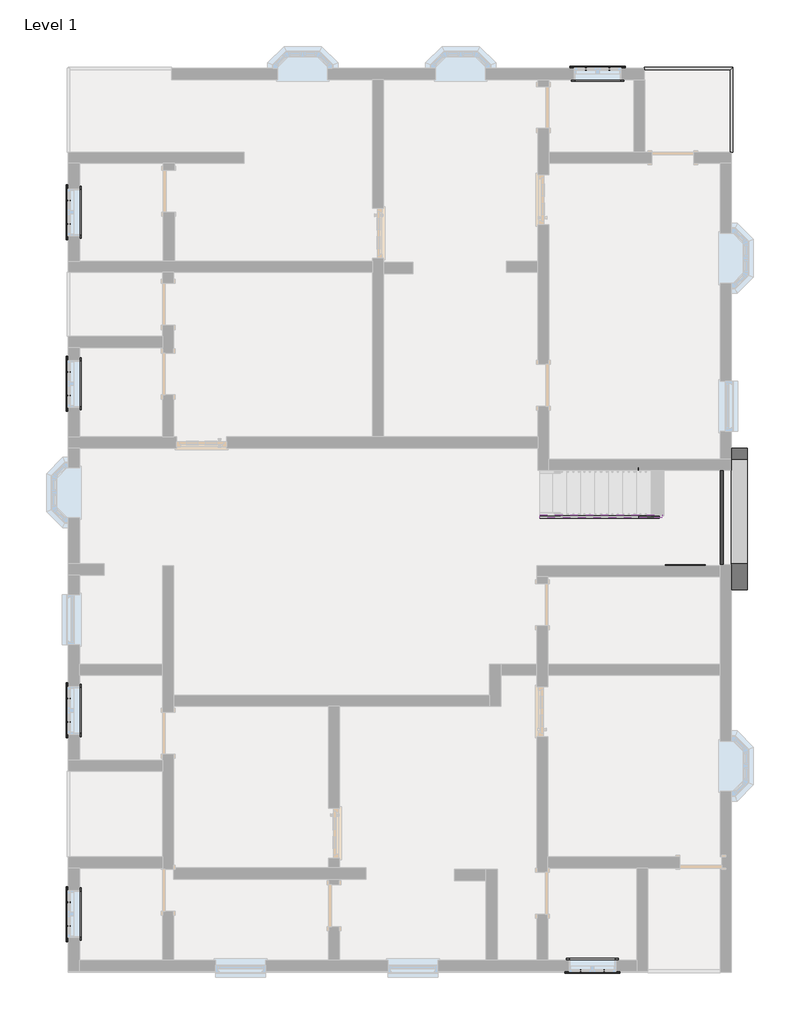
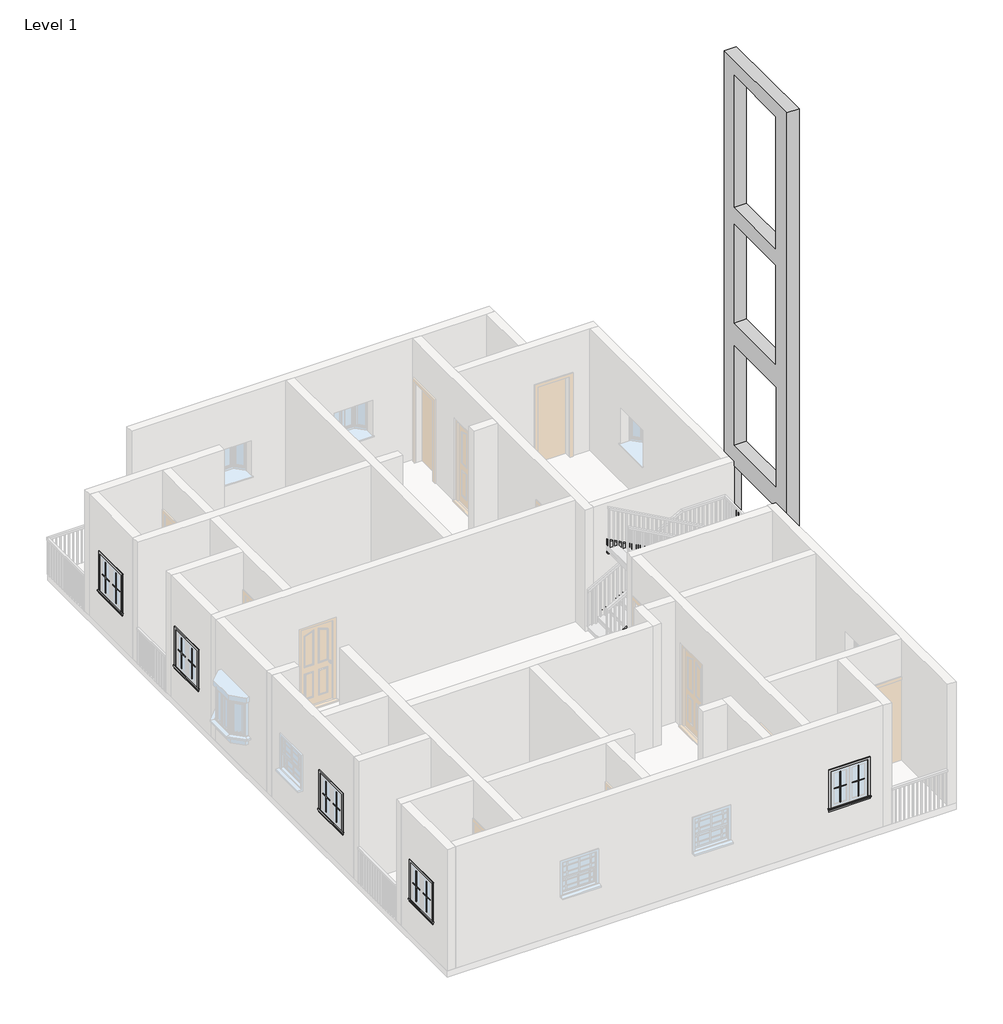
# One storey, part 4 of 4: 25 proxies, 5 members, 1 railing.
"""IFC4 building model written with IfcOpenShell, lengths in millimetres."""

from ifc_helpers import new_model, si_unit, frame, origin, origin_with_axes, place, context, project, spatial, polyline, outline, extrude, faceted_brep, transform, mapped, element, save
from components import generic_models_1_generic_models_1_8cf75778, muntin_pattern_2x2_muntin_pattern_2x2_b3fe6957, muntin_pattern_2x2_muntin_pattern_2x2_3e0ecaf2, trim_window_exterior_flat_with_sill_41619996, trim_window_interior_flat_picture_frame_51c85655

model = new_model("IFC4")

# Units and contexts
model_context = context("Model", 3, world=origin())
ifc_project = project(units=[si_unit("LENGTHUNIT", "METRE", prefix="MILLI")], contexts=[model_context])

# Site, building, storey
site = spatial("IfcSite", under=ifc_project)
building = spatial("IfcBuilding", under=site)
storey = spatial("IfcBuildingStorey", under=building, Name="Level 1", Elevation=0.0)

# Proxies
placement = place(None, origin())
generic_models_1_generic_models_1_shape = generic_models_1_generic_models_1_8cf75778(model_context)
element("IfcBuildingElementProxy", 1, Name="Generic Models 1 : Generic Models 1", ObjectType="Generic Models 1 : Generic Models 1", at=placement, inside=storey, context=model_context, shape_type="MappedRepresentation", body=[
    mapped(generic_models_1_generic_models_1_shape, transform((0.0, 0.0, 0.0), x_axis=(1.0, 0.0, 0.0), y_axis=(0.0, 1.0, 0.0), z_axis=(0.0, 0.0, 1.0))),
])
muntin_pattern_2x2_muntin_pattern_2x2_shape = muntin_pattern_2x2_muntin_pattern_2x2_b3fe6957(model_context)
element("IfcBuildingElementProxy", 2, Name="Muntin Pattern_2x2 : Muntin Pattern_2x2", ObjectType="Muntin Pattern_2x2 : Muntin Pattern_2x2", at=placement, inside=storey, context=model_context, shape_type="MappedRepresentation", body=[
    mapped(muntin_pattern_2x2_muntin_pattern_2x2_shape, transform((-7038.4808717, 5489.0318597, 984.25), x_axis=(0.0, 1.0, 0.0), y_axis=(-1.0, 0.0, 0.0), z_axis=(0.0, 0.0, 1.0))),
])
element("IfcBuildingElementProxy", 3, Name="Muntin Pattern_2x2 : Muntin Pattern_2x2", ObjectType="Muntin Pattern_2x2 : Muntin Pattern_2x2", at=placement, inside=storey, context=model_context, shape_type="MappedRepresentation", body=[
    mapped(muntin_pattern_2x2_muntin_pattern_2x2_shape, transform((-7038.4808717, 2366.9422293, 984.25), x_axis=(0.0, 1.0, 0.0), y_axis=(-1.0, 0.0, 0.0), z_axis=(0.0, 0.0, 1.0))),
])
element("IfcBuildingElementProxy", 4, Name="Muntin Pattern_2x2 : Muntin Pattern_2x2", ObjectType="Muntin Pattern_2x2 : Muntin Pattern_2x2", at=placement, inside=storey, context=model_context, shape_type="MappedRepresentation", body=[
    mapped(muntin_pattern_2x2_muntin_pattern_2x2_shape, transform((2376.9816283, 8312.1297293, 984.25), x_axis=(1.0, 0.0, 0.0), y_axis=(0.0, 1.0, 0.0), z_axis=(0.0, 0.0, 1.0))),
])
element("IfcBuildingElementProxy", 5, Name="Muntin Pattern_2x2 : Muntin Pattern_2x2", ObjectType="Muntin Pattern_2x2 : Muntin Pattern_2x2", at=placement, inside=storey, context=model_context, shape_type="MappedRepresentation", body=[
    mapped(muntin_pattern_2x2_muntin_pattern_2x2_shape, transform((2710.3566283, -8102.6202707, 984.25), x_axis=(-1.0, 0.0, 0.0), y_axis=(0.0, -1.0, 0.0), z_axis=(0.0, 0.0, 1.0))),
])
element("IfcBuildingElementProxy", 6, Name="Muntin Pattern_2x2 : Muntin Pattern_2x2", ObjectType="Muntin Pattern_2x2 : Muntin Pattern_2x2", at=placement, inside=storey, context=model_context, shape_type="MappedRepresentation", body=[
    mapped(muntin_pattern_2x2_muntin_pattern_2x2_shape, transform((-7038.4808717, -7285.0577707, 984.25), x_axis=(0.0, 1.0, 0.0), y_axis=(-1.0, 0.0, 0.0), z_axis=(0.0, 0.0, 1.0))),
])
element("IfcBuildingElementProxy", 7, Name="Muntin Pattern_2x2 : Muntin Pattern_2x2", ObjectType="Muntin Pattern_2x2 : Muntin Pattern_2x2", at=placement, inside=storey, context=model_context, shape_type="MappedRepresentation", body=[
    mapped(muntin_pattern_2x2_muntin_pattern_2x2_shape, transform((-7038.4808717, -3576.6577707, 984.25), x_axis=(0.0, 1.0, 0.0), y_axis=(-1.0, 0.0, 0.0), z_axis=(0.0, 0.0, 1.0))),
])
muntin_pattern_2x2_muntin_pattern_2x2_2_shape = muntin_pattern_2x2_muntin_pattern_2x2_3e0ecaf2(model_context)
element("IfcBuildingElementProxy", 8, Name="Muntin Pattern_2x2 : Muntin Pattern_2x2", ObjectType="Muntin Pattern_2x2 : Muntin Pattern_2x2", at=placement, inside=storey, context=model_context, shape_type="MappedRepresentation", body=[
    mapped(muntin_pattern_2x2_muntin_pattern_2x2_2_shape, transform((-7038.4808717, 5917.6568597, 984.25), x_axis=(0.0, -1.0, 0.0), y_axis=(1.0, 0.0, 0.0), z_axis=(0.0, 0.0, 1.0))),
])
element("IfcBuildingElementProxy", 9, Name="Muntin Pattern_2x2 : Muntin Pattern_2x2", ObjectType="Muntin Pattern_2x2 : Muntin Pattern_2x2", at=placement, inside=storey, context=model_context, shape_type="MappedRepresentation", body=[
    mapped(muntin_pattern_2x2_muntin_pattern_2x2_2_shape, transform((-7038.4808717, 2795.5672293, 984.25), x_axis=(0.0, -1.0, 0.0), y_axis=(1.0, 0.0, 0.0), z_axis=(0.0, 0.0, 1.0))),
])
element("IfcBuildingElementProxy", 10, Name="Muntin Pattern_2x2 : Muntin Pattern_2x2", ObjectType="Muntin Pattern_2x2 : Muntin Pattern_2x2", at=placement, inside=storey, context=model_context, shape_type="MappedRepresentation", body=[
    mapped(muntin_pattern_2x2_muntin_pattern_2x2_2_shape, transform((2805.6066283, 8312.1297293, 984.25), x_axis=(-1.0, 0.0, 0.0), y_axis=(0.0, -1.0, 0.0), z_axis=(0.0, 0.0, 1.0))),
])
element("IfcBuildingElementProxy", 11, Name="Muntin Pattern_2x2 : Muntin Pattern_2x2", ObjectType="Muntin Pattern_2x2 : Muntin Pattern_2x2", at=placement, inside=storey, context=model_context, shape_type="MappedRepresentation", body=[
    mapped(muntin_pattern_2x2_muntin_pattern_2x2_2_shape, transform((2281.7316283, -8102.6202707, 984.25), x_axis=(1.0, 0.0, 0.0), y_axis=(0.0, 1.0, 0.0), z_axis=(0.0, 0.0, 1.0))),
])
element("IfcBuildingElementProxy", 12, Name="Muntin Pattern_2x2 : Muntin Pattern_2x2", ObjectType="Muntin Pattern_2x2 : Muntin Pattern_2x2", at=placement, inside=storey, context=model_context, shape_type="MappedRepresentation", body=[
    mapped(muntin_pattern_2x2_muntin_pattern_2x2_2_shape, transform((-7038.4808717, -6856.4327707, 984.25), x_axis=(0.0, -1.0, 0.0), y_axis=(1.0, 0.0, 0.0), z_axis=(0.0, 0.0, 1.0))),
])
element("IfcBuildingElementProxy", 13, Name="Muntin Pattern_2x2 : Muntin Pattern_2x2", ObjectType="Muntin Pattern_2x2 : Muntin Pattern_2x2", at=placement, inside=storey, context=model_context, shape_type="MappedRepresentation", body=[
    mapped(muntin_pattern_2x2_muntin_pattern_2x2_2_shape, transform((-7038.4808717, -3148.0327707, 984.25), x_axis=(0.0, -1.0, 0.0), y_axis=(1.0, 0.0, 0.0), z_axis=(0.0, 0.0, 1.0))),
])
trim_window_exterior_flat_with_sill_shape = trim_window_exterior_flat_with_sill_41619996(model_context)
element("IfcBuildingElementProxy", 14, Name="Trim-Window-Exterior-Flat : with Sill", ObjectType="Trim-Window-Exterior-Flat : with Sill", at=placement, inside=storey, context=model_context, shape_type="MappedRepresentation", body=[
    mapped(trim_window_exterior_flat_with_sill_shape, transform((-7048.0058717, 5703.3443597, 1828.8), x_axis=(0.0, -1.0, 0.0), y_axis=(0.0, 0.0, 1.0), z_axis=(-1.0, 0.0, 0.0))),
])
element("IfcBuildingElementProxy", 15, Name="Trim-Window-Exterior-Flat : with Sill", ObjectType="Trim-Window-Exterior-Flat : with Sill", at=placement, inside=storey, context=model_context, shape_type="MappedRepresentation", body=[
    mapped(trim_window_exterior_flat_with_sill_shape, transform((-7048.0058717, 2581.2547293, 1828.8), x_axis=(0.0, -1.0, 0.0), y_axis=(0.0, 0.0, 1.0), z_axis=(-1.0, 0.0, 0.0))),
])
element("IfcBuildingElementProxy", 16, Name="Trim-Window-Exterior-Flat : with Sill", ObjectType="Trim-Window-Exterior-Flat : with Sill", at=placement, inside=storey, context=model_context, shape_type="MappedRepresentation", body=[
    mapped(trim_window_exterior_flat_with_sill_shape, transform((2591.2941283, 8321.6547293, 1828.8), x_axis=(-1.0, 0.0, 0.0), y_axis=(0.0, 0.0, 1.0), z_axis=(0.0, 1.0, 0.0))),
])
element("IfcBuildingElementProxy", 17, Name="Trim-Window-Exterior-Flat : with Sill", ObjectType="Trim-Window-Exterior-Flat : with Sill", at=placement, inside=storey, context=model_context, shape_type="MappedRepresentation", body=[
    mapped(trim_window_exterior_flat_with_sill_shape, transform((2496.0441283, -8112.1452707, 1828.8), x_axis=(1.0, 0.0, 0.0), y_axis=(0.0, 0.0, 1.0), z_axis=(0.0, -1.0, 0.0))),
])
element("IfcBuildingElementProxy", 18, Name="Trim-Window-Exterior-Flat : with Sill", ObjectType="Trim-Window-Exterior-Flat : with Sill", at=placement, inside=storey, context=model_context, shape_type="MappedRepresentation", body=[
    mapped(trim_window_exterior_flat_with_sill_shape, transform((-7048.0058717, -7070.7452707, 1828.8), x_axis=(0.0, -1.0, 0.0), y_axis=(0.0, 0.0, 1.0), z_axis=(-1.0, 0.0, 0.0))),
])
element("IfcBuildingElementProxy", 19, Name="Trim-Window-Exterior-Flat : with Sill", ObjectType="Trim-Window-Exterior-Flat : with Sill", at=placement, inside=storey, context=model_context, shape_type="MappedRepresentation", body=[
    mapped(trim_window_exterior_flat_with_sill_shape, transform((-7048.0058717, -3362.3452707, 1828.8), x_axis=(0.0, -1.0, 0.0), y_axis=(0.0, 0.0, 1.0), z_axis=(-1.0, 0.0, 0.0))),
])
trim_window_interior_flat_picture_frame_shape = trim_window_interior_flat_picture_frame_51c85655(model_context)
element("IfcBuildingElementProxy", 20, Name="Trim-Window-Interior-Flat : Picture Frame", ObjectType="Trim-Window-Interior-Flat : Picture Frame", at=placement, inside=storey, context=model_context, shape_type="MappedRepresentation", body=[
    mapped(trim_window_interior_flat_picture_frame_shape, transform((-6844.8058717, 5703.3443597, 1828.8), x_axis=(0.0, 1.0, 0.0), y_axis=(0.0, 0.0, 1.0), z_axis=(1.0, 0.0, 0.0))),
])
element("IfcBuildingElementProxy", 21, Name="Trim-Window-Interior-Flat : Picture Frame", ObjectType="Trim-Window-Interior-Flat : Picture Frame", at=placement, inside=storey, context=model_context, shape_type="MappedRepresentation", body=[
    mapped(trim_window_interior_flat_picture_frame_shape, transform((-6844.8058717, 2581.2547293, 1828.8), x_axis=(0.0, 1.0, 0.0), y_axis=(0.0, 0.0, 1.0), z_axis=(1.0, 0.0, 0.0))),
])
element("IfcBuildingElementProxy", 22, Name="Trim-Window-Interior-Flat : Picture Frame", ObjectType="Trim-Window-Interior-Flat : Picture Frame", at=placement, inside=storey, context=model_context, shape_type="MappedRepresentation", body=[
    mapped(trim_window_interior_flat_picture_frame_shape, transform((2591.2941283, 8118.4547293, 1828.8), x_axis=(1.0, 0.0, 0.0), y_axis=(0.0, 0.0, 1.0), z_axis=(0.0, -1.0, 0.0))),
])
element("IfcBuildingElementProxy", 23, Name="Trim-Window-Interior-Flat : Picture Frame", ObjectType="Trim-Window-Interior-Flat : Picture Frame", at=placement, inside=storey, context=model_context, shape_type="MappedRepresentation", body=[
    mapped(trim_window_interior_flat_picture_frame_shape, transform((2496.0441283, -7908.9452707, 1828.8), x_axis=(-1.0, 0.0, 0.0), y_axis=(0.0, 0.0, 1.0), z_axis=(0.0, 1.0, 0.0))),
])
element("IfcBuildingElementProxy", 24, Name="Trim-Window-Interior-Flat : Picture Frame", ObjectType="Trim-Window-Interior-Flat : Picture Frame", at=placement, inside=storey, context=model_context, shape_type="MappedRepresentation", body=[
    mapped(trim_window_interior_flat_picture_frame_shape, transform((-6844.8058717, -7070.7452707, 1828.8), x_axis=(0.0, 1.0, 0.0), y_axis=(0.0, 0.0, 1.0), z_axis=(1.0, 0.0, 0.0))),
])
element("IfcBuildingElementProxy", 25, Name="Trim-Window-Interior-Flat : Picture Frame", ObjectType="Trim-Window-Interior-Flat : Picture Frame", at=placement, inside=storey, context=model_context, shape_type="MappedRepresentation", body=[
    mapped(trim_window_interior_flat_picture_frame_shape, transform((-6844.8058717, -3362.3452707, 1828.8), x_axis=(0.0, 1.0, 0.0), y_axis=(0.0, 0.0, 1.0), z_axis=(1.0, 0.0, 0.0))),
])

# Members
element("IfcMember", 26, ObjectType="Stringer - 2\" Width", at=placement, inside=storey, context=model_context, shape_type="SweptSolid", body=[
    extrude(outline(polyline([(210.6757607, 1537.1941283), (0.0, 1537.1941283), (0.0, 1786.1766781), (1447.8, 4407.1563102), (1447.8, 3776.7834593), (210.6757607, 1537.1941283)])), frame((0.0, 1006.4547293, 0.0), z_axis=(0.0, 1.0, 0.0), x_axis=(0.0, 0.0, 1.0)), (0.0, 0.0, 1.0), 50.8),
])
element("IfcMember", 27, ObjectType="Stringer - 2\" Width", at=placement, inside=storey, context=model_context, shape_type="SweptSolid", body=[
    extrude(outline(polyline([(4826.4941283, 1057.2547293), (4877.2941283, 1057.2547293), (4877.2941283, -714.2964201), (4826.4941283, -714.2964201), (4826.4941283, 1057.2547293)])), frame((0.0, 0.0, 1143.0), z_axis=(0.0, 0.0, 1.0), x_axis=(1.0, 0.0, 0.0)), (0.0, 0.0, 1.0), 304.8),
])
element("IfcMember", 28, ObjectType="Stringer - 2\" Width", at=placement, inside=storey, context=model_context, shape_type="SweptSolid", body=[
    extrude(outline(polyline([(1143.0, 4555.0346706), (2810.0215532, 1537.1941283), (2461.8106009, 1537.1941283), (1143.0, 3924.6618197), (1143.0, 4555.0346706)])), frame((0.0, -765.0964201, 0.0), z_axis=(0.0, 1.0, 0.0), x_axis=(0.0, 0.0, 1.0)), (0.0, 0.0, 1.0), 50.8),
])
element("IfcMember", 29, ObjectType="Stringer - 2\" Width", at=placement, inside=storey, context=model_context, shape_type="SweptSolid", body=[
    extrude(outline(polyline([(210.6757607, 1537.1941283), (0.0, 1537.1941283), (0.0, 1786.1766781), (1065.4963497, 3715.0648053), (1413.7073019, 3715.0648053), (210.6757607, 1537.1941283)])), frame((0.0, 130.1547293, 0.0), z_axis=(0.0, 1.0, 0.0), x_axis=(0.0, 0.0, 1.0)), (0.0, 0.0, 1.0), 50.8),
])
element("IfcMember", 30, ObjectType="Stringer - 2\" Width", at=placement, inside=storey, context=model_context, shape_type="SweptSolid", body=[
    extrude(outline(polyline([(1230.7177047, 3765.8648053), (1578.928657, 3765.8648053), (2810.0215532, 1537.1941283), (2461.8106009, 1537.1941283), (1230.7177047, 3765.8648053)])), frame((0.0, 142.8547293, 0.0), z_axis=(0.0, 1.0, 0.0), x_axis=(0.0, 0.0, 1.0)), (0.0, 0.0, 1.0), 50.8),
])

# Railing
element("IfcRailing", 31, ObjectType="Handrail - Rectangular", at=placement, inside=storey, context=model_context, shape_type="SolidModel", body=[
    faceted_brep([(3442.1941283, 8347.0547293, 914.4), (3442.1941283, 8347.0547293, 863.6), (3442.1941283, 8296.2547293, 863.6), (3442.1941283, 8296.2547293, 914.4), (5055.0941283, 8347.0547293, 914.4), (5055.0941283, 8347.0547293, 863.6), (5004.2941283, 8296.2547293, 863.6), (5004.2941283, 8296.2547293, 914.4), (5055.0941283, 6797.6547293, 914.4), (5004.2941283, 6797.6547293, 914.4), (5004.2941283, 6797.6547293, 863.6), (5055.0941283, 6797.6547293, 863.6)], [[[0, 1, 2, 3]], [[1, 0, 4, 5]], [[2, 1, 5, 6]], [[3, 2, 6, 7]], [[0, 3, 7, 4]], [[8, 9, 10, 11]], [[5, 4, 8, 11]], [[6, 5, 11, 10]], [[7, 6, 10, 9]], [[4, 7, 9, 8]]]),
    extrude(outline(polyline([(5020.1691283, 6908.7797293), (5039.2191283, 6908.7797293), (5039.2191283, 6889.7297293), (5020.1691283, 6889.7297293), (5020.1691283, 6908.7797293)])), origin_with_axes(), (0.0, 0.0, 1.0), 863.6),
    extrude(outline(polyline([(5020.1691283, 7010.3797293), (5039.2191283, 7010.3797293), (5039.2191283, 6991.3297293), (5020.1691283, 6991.3297293), (5020.1691283, 7010.3797293)])), origin_with_axes(), (0.0, 0.0, 1.0), 863.6),
    extrude(outline(polyline([(5020.1691283, 7111.9797293), (5039.2191283, 7111.9797293), (5039.2191283, 7092.9297293), (5020.1691283, 7092.9297293), (5020.1691283, 7111.9797293)])), origin_with_axes(), (0.0, 0.0, 1.0), 863.6),
    extrude(outline(polyline([(5020.1691283, 7213.5797293), (5039.2191283, 7213.5797293), (5039.2191283, 7194.5297293), (5020.1691283, 7194.5297293), (5020.1691283, 7213.5797293)])), origin_with_axes(), (0.0, 0.0, 1.0), 863.6),
    extrude(outline(polyline([(5020.1691283, 7315.1797293), (5039.2191283, 7315.1797293), (5039.2191283, 7296.1297293), (5020.1691283, 7296.1297293), (5020.1691283, 7315.1797293)])), origin_with_axes(), (0.0, 0.0, 1.0), 863.6),
    extrude(outline(polyline([(5020.1691283, 7416.7797293), (5039.2191283, 7416.7797293), (5039.2191283, 7397.7297293), (5020.1691283, 7397.7297293), (5020.1691283, 7416.7797293)])), origin_with_axes(), (0.0, 0.0, 1.0), 863.6),
    extrude(outline(polyline([(5020.1691283, 7518.3797293), (5039.2191283, 7518.3797293), (5039.2191283, 7499.3297293), (5020.1691283, 7499.3297293), (5020.1691283, 7518.3797293)])), origin_with_axes(), (0.0, 0.0, 1.0), 863.6),
    extrude(outline(polyline([(5020.1691283, 7619.9797293), (5039.2191283, 7619.9797293), (5039.2191283, 7600.9297293), (5020.1691283, 7600.9297293), (5020.1691283, 7619.9797293)])), origin_with_axes(), (0.0, 0.0, 1.0), 863.6),
    extrude(outline(polyline([(5020.1691283, 7721.5797293), (5039.2191283, 7721.5797293), (5039.2191283, 7702.5297293), (5020.1691283, 7702.5297293), (5020.1691283, 7721.5797293)])), origin_with_axes(), (0.0, 0.0, 1.0), 863.6),
    extrude(outline(polyline([(5020.1691283, 7823.1797293), (5039.2191283, 7823.1797293), (5039.2191283, 7804.1297293), (5020.1691283, 7804.1297293), (5020.1691283, 7823.1797293)])), origin_with_axes(), (0.0, 0.0, 1.0), 863.6),
    extrude(outline(polyline([(5020.1691283, 7924.7797293), (5039.2191283, 7924.7797293), (5039.2191283, 7905.7297293), (5020.1691283, 7905.7297293), (5020.1691283, 7924.7797293)])), origin_with_axes(), (0.0, 0.0, 1.0), 863.6),
    extrude(outline(polyline([(5020.1691283, 8026.3797293), (5039.2191283, 8026.3797293), (5039.2191283, 8007.3297293), (5020.1691283, 8007.3297293), (5020.1691283, 8026.3797293)])), origin_with_axes(), (0.0, 0.0, 1.0), 863.6),
    extrude(outline(polyline([(5020.1691283, 8127.9797293), (5039.2191283, 8127.9797293), (5039.2191283, 8108.9297293), (5020.1691283, 8108.9297293), (5020.1691283, 8127.9797293)])), origin_with_axes(), (0.0, 0.0, 1.0), 863.6),
    extrude(outline(polyline([(5020.1691283, 8229.5797293), (5039.2191283, 8229.5797293), (5039.2191283, 8210.5297293), (5020.1691283, 8210.5297293), (5020.1691283, 8229.5797293)])), origin_with_axes(), (0.0, 0.0, 1.0), 863.6),
    extrude(outline(polyline([(4956.6691283, 8312.1297293), (4956.6691283, 8331.1797293), (4975.7191283, 8331.1797293), (4975.7191283, 8312.1297293), (4956.6691283, 8312.1297293)])), origin_with_axes(), (0.0, 0.0, 1.0), 863.6),
    extrude(outline(polyline([(4855.0691283, 8312.1297293), (4855.0691283, 8331.1797293), (4874.1191283, 8331.1797293), (4874.1191283, 8312.1297293), (4855.0691283, 8312.1297293)])), origin_with_axes(), (0.0, 0.0, 1.0), 863.6),
    extrude(outline(polyline([(4753.4691283, 8312.1297293), (4753.4691283, 8331.1797293), (4772.5191283, 8331.1797293), (4772.5191283, 8312.1297293), (4753.4691283, 8312.1297293)])), origin_with_axes(), (0.0, 0.0, 1.0), 863.6),
    extrude(outline(polyline([(4651.8691283, 8312.1297293), (4651.8691283, 8331.1797293), (4670.9191283, 8331.1797293), (4670.9191283, 8312.1297293), (4651.8691283, 8312.1297293)])), origin_with_axes(), (0.0, 0.0, 1.0), 863.6),
    extrude(outline(polyline([(4550.2691283, 8312.1297293), (4550.2691283, 8331.1797293), (4569.3191283, 8331.1797293), (4569.3191283, 8312.1297293), (4550.2691283, 8312.1297293)])), origin_with_axes(), (0.0, 0.0, 1.0), 863.6),
    extrude(outline(polyline([(4448.6691283, 8312.1297293), (4448.6691283, 8331.1797293), (4467.7191283, 8331.1797293), (4467.7191283, 8312.1297293), (4448.6691283, 8312.1297293)])), origin_with_axes(), (0.0, 0.0, 1.0), 863.6),
    extrude(outline(polyline([(4347.0691283, 8312.1297293), (4347.0691283, 8331.1797293), (4366.1191283, 8331.1797293), (4366.1191283, 8312.1297293), (4347.0691283, 8312.1297293)])), origin_with_axes(), (0.0, 0.0, 1.0), 863.6),
    extrude(outline(polyline([(4245.4691283, 8312.1297293), (4245.4691283, 8331.1797293), (4264.5191283, 8331.1797293), (4264.5191283, 8312.1297293), (4245.4691283, 8312.1297293)])), origin_with_axes(), (0.0, 0.0, 1.0), 863.6),
    extrude(outline(polyline([(4143.8691283, 8312.1297293), (4143.8691283, 8331.1797293), (4162.9191283, 8331.1797293), (4162.9191283, 8312.1297293), (4143.8691283, 8312.1297293)])), origin_with_axes(), (0.0, 0.0, 1.0), 863.6),
    extrude(outline(polyline([(4042.2691283, 8312.1297293), (4042.2691283, 8331.1797293), (4061.3191283, 8331.1797293), (4061.3191283, 8312.1297293), (4042.2691283, 8312.1297293)])), origin_with_axes(), (0.0, 0.0, 1.0), 863.6),
    extrude(outline(polyline([(3940.6691283, 8312.1297293), (3940.6691283, 8331.1797293), (3959.7191283, 8331.1797293), (3959.7191283, 8312.1297293), (3940.6691283, 8312.1297293)])), origin_with_axes(), (0.0, 0.0, 1.0), 863.6),
    extrude(outline(polyline([(3839.0691283, 8312.1297293), (3839.0691283, 8331.1797293), (3858.1191283, 8331.1797293), (3858.1191283, 8312.1297293), (3839.0691283, 8312.1297293)])), origin_with_axes(), (0.0, 0.0, 1.0), 863.6),
    extrude(outline(polyline([(3737.4691283, 8312.1297293), (3737.4691283, 8331.1797293), (3756.5191283, 8331.1797293), (3756.5191283, 8312.1297293), (3737.4691283, 8312.1297293)])), origin_with_axes(), (0.0, 0.0, 1.0), 863.6),
    extrude(outline(polyline([(3635.8691283, 8312.1297293), (3635.8691283, 8331.1797293), (3654.9191283, 8331.1797293), (3654.9191283, 8312.1297293), (3635.8691283, 8312.1297293)])), origin_with_axes(), (0.0, 0.0, 1.0), 863.6),
    extrude(outline(polyline([(3534.2691283, 8312.1297293), (3534.2691283, 8331.1797293), (3553.3191283, 8331.1797293), (3553.3191283, 8312.1297293), (3534.2691283, 8312.1297293)])), origin_with_axes(), (0.0, 0.0, 1.0), 863.6),
    extrude(outline(polyline([(5020.1691283, 8312.1297293), (5020.1691283, 8331.1797293), (5039.2191283, 8331.1797293), (5039.2191283, 8312.1297293), (5020.1691283, 8312.1297293)])), origin_with_axes(), (0.0, 0.0, 1.0), 863.6),
    extrude(outline(polyline([(5020.1691283, 6816.7047293), (5039.2191283, 6816.7047293), (5039.2191283, 6797.6547293), (5020.1691283, 6797.6547293), (5020.1691283, 6816.7047293)])), origin_with_axes(), (0.0, 0.0, 1.0), 863.6),
    extrude(outline(polyline([(3442.1941283, 8312.1297293), (3442.1941283, 8331.1797293), (3461.2441283, 8331.1797293), (3461.2441283, 8312.1297293), (3442.1941283, 8312.1297293)])), origin_with_axes(), (0.0, 0.0, 1.0), 863.6),
])

save(model, "model.ifc")

# Revit data of these elements
# Type "Muntin Pattern_2x2 : Muntin Pattern_2x2"
#   Width [instance default] = 4' - 0"
#   Thickness = 0' - 0 1/2"
#   Height [instance default] = 4' - 0"
#   Distance = 0' - 0 3/4"
#   Interior Material [instance default] = none
#   Exterior Material [instance default] = none
#   Default Elevation = 0
# Type "Trim-Window-Exterior-Flat : with Sill"
#   Trim Width = 0' - 2 1/4"
#   Trim Thickness_Picture Frame = 0' - 1 1/4"
#   Trim Thickness_with Sill = 0' - 0 3/4"
#   Sill Thickness = 0' - 1 1/4"
#   Opening Width [instance default] = 2' - 0"
#   Opening Height [instance default] = 3' - 0"
#   Default Elevation = 4' - 0"
#   Sill = yes
#   Picture Frame = no
#   Trim Material [instance default] = none
# Type "Trim-Window-Interior-Flat : Picture Frame"
#   Trim Thickness_Picture Frame = 0' - 1 1/4"
#   Trim Width = 0' - 2 1/4"
#   Trim Thickness_with Sill = 0' - 0 3/4"
#   Sill Thickness = 0' - 1 1/4"
#   Opening Width [instance default] = 2' - 0"
#   Opening Height [instance default] = 3' - 0"
#   Default Elevation = 4' - 0"
#   Sill = no
#   Picture Frame = yes
#   Trim Material [instance default] = none
# Type "Handrail - Rectangular"
#   Assembly Code = "C2010400"
#   built-in parameter 1008612 = 0.0416667 (stored number, unit not read)
#   built-in parameter 1008611 = 0.0416667 (stored number, unit not read)
#   built-in parameter 1008609 = 0.333333 (stored number, unit not read)
#   built-in parameter 1008604 = 0.166667 (stored number, unit not read)
#   built-in parameter 1008603 = 0.166667 (stored number, unit not read)
#   Railing Height = 3' - 0"
#   built-in parameter 1008630 = 2
#   built-in parameter 1008610 = 2
#   built-in parameter 1008618 = Baluster - Square : 3/4"
# Element 1 (IfcBuildingElementProxy, "Generic Models 1 : Generic Models 1")
#   Phase Created = New Construction
#   Materials on its faces: "Acoustic Ceiling Tile 24 x 24", "Door - Frame"
# Elements 2, 3, 4, 5, 6, 7, 8, 9, 10, 11, 12, 13 (IfcBuildingElementProxy, "Muntin Pattern_2x2 : Muntin Pattern_2x2")
#   Width = 0' - 11 5/8"
#   Height = 2' - 6 1/2"
#   Interior Material = Wood - Stained
#   Exterior Material = Clad - White
#   Phase Created = New Construction
#   Materials on its faces: "Clad - White", "Wood - Stained"
# Elements 14, 15, 16, 17, 18, 19 (IfcBuildingElementProxy, "Trim-Window-Exterior-Flat : with Sill")
#   Opening Width = 2' - 10"
#   Opening Height = 3' - 0"
#   Trim Material = Clad - White
#   Phase Created = New Construction
#   Materials on its faces: "Clad - White"
# Elements 20, 21, 22, 23, 24, 25 (IfcBuildingElementProxy, "Trim-Window-Interior-Flat : Picture Frame")
#   Opening Width = 2' - 10"
#   Opening Height = 3' - 0"
#   Trim Material = Wood - Stained
#   Phase Created = New Construction
#   Materials on its faces: "Wood - Stained"
# Elements 26, 28, 29, 30 (IfcMember, "Stringer - 2\" Width")
#   Phase Created = New Construction
# Element 27 (IfcMember, "Stringer - 2\" Width")
#   Phase Created = New Construction
#   Materials on its faces: "Render Material 41-165-0"
# Element 31 (IfcRailing, "Handrail - Rectangular")
#   Phase Created = New Construction
# Materials
#   "Acoustic Ceiling Tile 24 x 24": class "Generic", colour RGB 232 232 232, transparency 0, Description = "Acoustic Ceiling Tile 24 x 24", Cost = 0
#   "Door - Frame": colour RGB 118 70 51, transparency 0, Cost = 0
#   "Clad - White": class "Wood", colour RGB 242 242 238, transparency 0, Cost = 0
#   "Wood - Stained": class "Wood", colour RGB 224 178 126, transparency 0, Cost = 0
#   "Render Material 41-165-0": colour RGB 41 165 0, transparency 0
